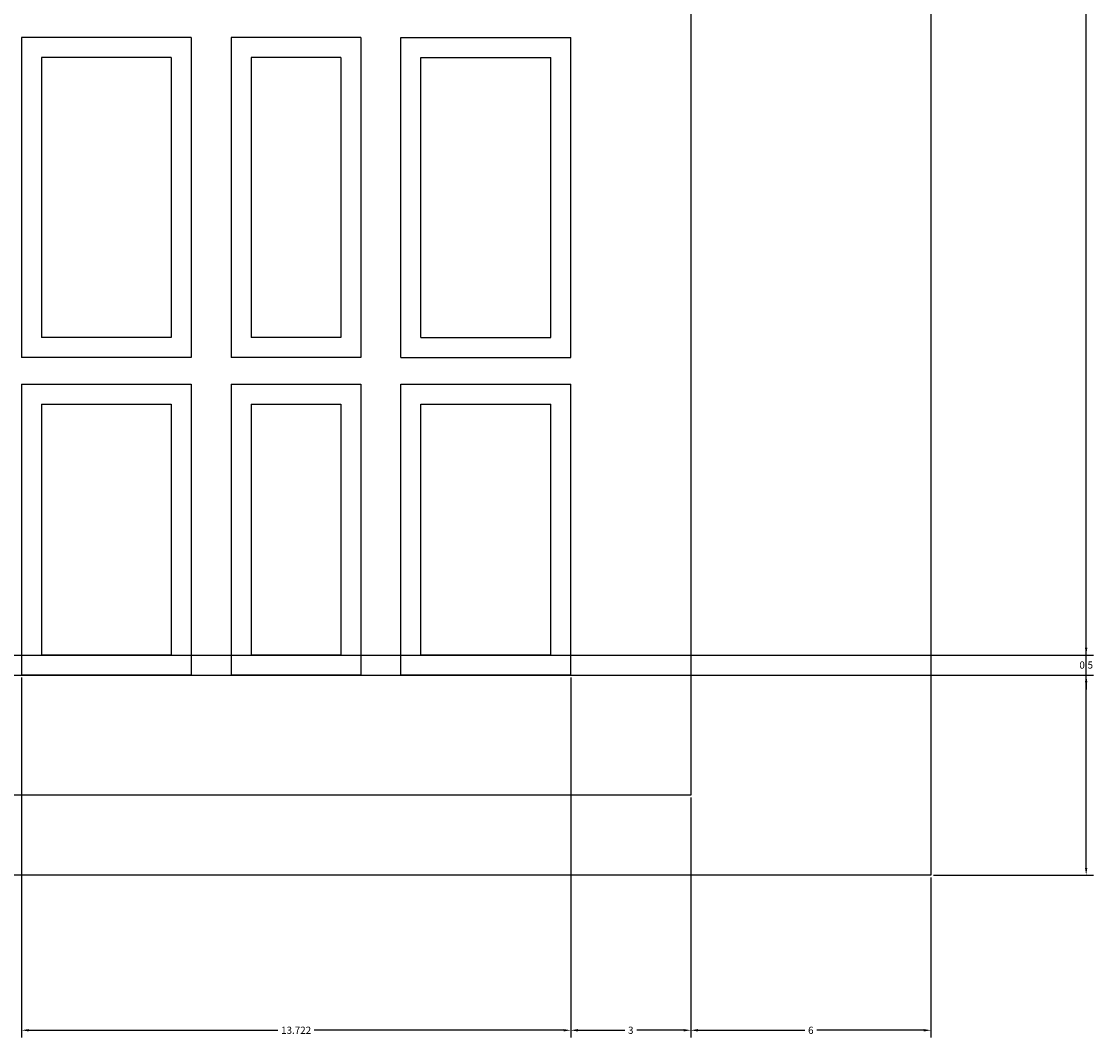
# Model space of a CAD drawing. Units: inches. Extents: x 12532.3 to 12594.9, y 6967.5 to 7063.
# Tile 4 of 9: x 12566.2 to 12593.1, y 6967.5 to 6992.9. Entities that reach past the tile are written whole.
import ezdxf

# ---------------------------------------------------------------- set-up
doc = ezdxf.new("R2010")
doc.units = ezdxf.units.IN
doc.header["$MEASUREMENT"] = 0
doc.header["$PDMODE"] = 98
doc.layers.add('A-ANNO-DIMS', color=2, linetype='Continuous', lineweight=18)
doc.layers.add('A-DOOR', color=4, linetype='Continuous', lineweight=25)
doc.styles.get("Standard").update_dxf_attribs({"font": 'arial.ttf'})
doc.dimstyles.get("Standard").update_dxf_attribs({"dimtxt": 0.18, "dimasz": 0.18, "dimexe": 0.18, "dimexo": 0.0625, "dimgap": 0.09, "dimtad": 0, "dimtih": 1, "dimtoh": 1, "dimdec": 4, "dimzin": 0, "dimdsep": 46, "dimtxsty": 'Standard', "dimcen": 0.09, "dimadec": 0, "dimazin": 0, "dimtfac": 1, "dimtdec": 4, "dimtofl": 0, "dimtmove": 0, "dimatfit": 3, "dimfxl": 1, "dimtolj": 1, "dimtzin": 0, "dimarcsym": 0})

# ---------------------------------------------------------------- blocks, each defined once
blk = doc.blocks.new('DOOR-PANEL-3_2x7_3')
for p, q in [((0, 7.273), (0, 0)), ((0, 7.273), (3.24, 7.273)), ((3.24, 7.273), (3.24, 0)), ((0.5, 6.773), (0.5, 0.5)), ((0.5, 6.773), (2.74, 6.773)), ((2.74, 6.773), (2.74, 0.5)), ((2.74, 0.5), (0.5, 0.5)), ((3.24, 0), (0, 0))]:
    blk.add_line(p, q)
blk = doc.blocks.new('DOOR-PANEL-4_2x7_3')
for p, q in [((0, 7.273), (0, 0)), ((0, 7.273), (4.241, 7.273)), ((4.241, 7.273), (4.241, 0)), ((0.5, 6.773), (0.5, 0.5)), ((0.5, 6.773), (3.741, 6.773)), ((3.741, 6.773), (3.741, 0.5)), ((3.741, 0.5), (0.5, 0.5)), ((4.241, 0), (0, 0))]:
    blk.add_line(p, q)
blk = doc.blocks.new('DOOR-PANEL-4_2x8_0')
for p, q in [((4.241, 8.003), (0, 8.003)), ((0, 8.003), (0, 0)), ((4.241, 8.003), (4.241, 0)), ((3.741, 7.503), (0.5, 7.503)), ((0.5, 7.503), (0.5, 0.5)), ((3.741, 7.503), (3.741, 0.5)), ((3.741, 0.5), (0.5, 0.5)), ((4.241, 0), (0, 0))]:
    blk.add_line(p, q)
blk = doc.blocks.new('DOOR-PANEL-3_2x8_0')
for p, q in [((3.24, 8.003), (0, 8.003)), ((0, 8.003), (0, 0)), ((3.24, 8.003), (3.24, 0)), ((2.74, 7.503), (0.5, 7.503)), ((0.5, 7.503), (0.5, 0.5)), ((2.74, 7.503), (2.74, 0.5)), ((2.74, 0.5), (0.5, 0.5)), ((3.24, 0), (0, 0))]:
    blk.add_line(p, q)
blk = doc.blocks.new('*D32')
at = {"layer": 'A-ANNO-DIMS', "color": 0, "lineweight": -2, "transparency": 16777216}
for p, q in [((12588.956, 7020.929), (12592.954, 7020.929)), ((12592.774, 7020.749), (12592.774, 6996.445)), ((12592.774, 6971.777), (12592.774, 6996.081)), ((12588.956, 6971.597), (12592.954, 6971.597))]:
    blk.add_line(p, q, dxfattribs=at)
at = {"layer": 'A-ANNO-DIMS', "color": 0, "transparency": 16777216}
for points in [[(12592.744, 7020.749), (12592.804, 7020.749), (12592.774, 7020.929)], [(12592.744, 6971.777), (12592.804, 6971.777), (12592.774, 6971.597)]]:
    blk.add_solid(points, dxfattribs=at)
at = {"layer": 'Defpoints', "color": 0, "transparency": 16777216}
for p in [(12588.894, 7020.929), (12592.774, 7020.929), (12588.894, 6971.597)]:
    blk.add_point(p, dxfattribs=at)
at = {"layer": 'A-ANNO-DIMS', "color": 0, "transparency": 16777216, "insert": (12592.774, 6996.263), "char_height": 0.18, "attachment_point": 5}
blk.add_mtext('\\A1;49.33', dxfattribs=at)
blk = doc.blocks.new('*D38')
at = {"layer": 'A-ANNO-DIMS', "color": 0, "lineweight": -2, "transparency": 16777216}
for p, q in [((12566.172, 6976.534), (12566.172, 6967.537)), ((12579.894, 6976.534), (12579.894, 6967.537)), ((12566.352, 6967.717), (12572.579, 6967.717)), ((12579.714, 6967.717), (12573.487, 6967.717))]:
    blk.add_line(p, q, dxfattribs=at)
at = {"layer": 'A-ANNO-DIMS', "color": 0, "transparency": 16777216}
for points in [[(12566.352, 6967.747), (12566.352, 6967.687), (12566.172, 6967.717)], [(12579.714, 6967.747), (12579.714, 6967.687), (12579.894, 6967.717)]]:
    blk.add_solid(points, dxfattribs=at)
at = {"layer": 'Defpoints', "color": 0, "transparency": 16777216}
for p in [(12566.172, 6976.597), (12579.894, 6976.597), (12579.894, 6967.717)]:
    blk.add_point(p, dxfattribs=at)
at = {"layer": 'A-ANNO-DIMS', "color": 0, "transparency": 16777216, "insert": (12573.033, 6967.717), "char_height": 0.18, "attachment_point": 5}
blk.add_mtext('\\A1;13.722', dxfattribs=at)
blk = doc.blocks.new('*D39')
at = {"layer": 'A-ANNO-DIMS', "color": 0, "lineweight": -2, "transparency": 16777216}
for p, q in [((12579.894, 6976.534), (12579.894, 6967.537)), ((12582.894, 6973.534), (12582.894, 6967.537)), ((12580.074, 6967.717), (12581.245, 6967.717)), ((12582.714, 6967.717), (12581.543, 6967.717))]:
    blk.add_line(p, q, dxfattribs=at)
at = {"layer": 'A-ANNO-DIMS', "color": 0, "transparency": 16777216}
for points in [[(12580.074, 6967.747), (12580.074, 6967.687), (12579.894, 6967.717)], [(12582.714, 6967.747), (12582.714, 6967.687), (12582.894, 6967.717)]]:
    blk.add_solid(points, dxfattribs=at)
at = {"layer": 'Defpoints', "color": 0, "transparency": 16777216}
for p in [(12579.894, 6976.597), (12582.894, 6973.597), (12582.894, 6967.717)]:
    blk.add_point(p, dxfattribs=at)
at = {"layer": 'A-ANNO-DIMS', "color": 0, "transparency": 16777216, "insert": (12581.394, 6967.717), "char_height": 0.18, "attachment_point": 5}
blk.add_mtext('\\A1;3', dxfattribs=at)
blk = doc.blocks.new('*D40')
at = {"layer": 'A-ANNO-DIMS', "color": 0, "lineweight": -2, "transparency": 16777216}
for p, q in [((12582.893999, 6973.534253), (12582.893999, 6967.536753)), ((12588.893999, 6971.534253), (12588.893999, 6967.536753)), ((12583.073999, 6967.716753), (12585.744572, 6967.716753)), ((12588.713999, 6967.716753), (12586.043426, 6967.716753))]:
    blk.add_line(p, q, dxfattribs=at)
at = {"layer": 'A-ANNO-DIMS', "color": 0, "transparency": 16777216}
for points in [[(12583.073999, 6967.746753), (12583.073999, 6967.686753), (12582.893999, 6967.716753)], [(12588.713999, 6967.746753), (12588.713999, 6967.686753), (12588.893999, 6967.716753)]]:
    blk.add_solid(points, dxfattribs=at)
at = {"layer": 'Defpoints', "color": 0, "transparency": 16777216}
for p in [(12582.893999, 6973.596753), (12588.893999, 6971.596753), (12588.893999, 6967.716753)]:
    blk.add_point(p, dxfattribs=at)
at = {"layer": 'A-ANNO-DIMS', "color": 0, "transparency": 16777216, "insert": (12585.893999, 6967.716753), "char_height": 0.18, "attachment_point": 5}
blk.add_mtext('\\A1;6', dxfattribs=at)
blk = doc.blocks.new('*D61')
at = {"layer": 'A-ANNO-DIMS', "color": 0, "lineweight": -2, "transparency": 16777216}
for p, q in [((12592.773999, 6977.276753), (12592.773999, 6977.456753)), ((12558.734573, 6977.096753), (12592.953999, 6977.096753)), ((12559.234573, 6976.596753), (12592.953999, 6976.596753)), ((12592.773999, 6976.416753), (12592.773999, 6976.236753))]:
    blk.add_line(p, q, dxfattribs=at)
at = {"layer": 'A-ANNO-DIMS', "color": 0, "transparency": 16777216}
for points in [[(12592.743999, 6977.276753), (12592.803999, 6977.276753), (12592.773999, 6977.096753)], [(12592.743999, 6976.416753), (12592.803999, 6976.416753), (12592.773999, 6976.596753)]]:
    blk.add_solid(points, dxfattribs=at)
at = {"layer": 'Defpoints', "color": 0, "transparency": 16777216}
for p in [(12558.672073, 6977.096753), (12592.773999, 6977.096753), (12559.172073, 6976.596753)]:
    blk.add_point(p, dxfattribs=at)
at = {"layer": 'A-ANNO-DIMS', "color": 0, "transparency": 16777216, "insert": (12592.773999, 6976.846753), "char_height": 0.18, "attachment_point": 5}
blk.add_mtext('\\A1;0.5', dxfattribs=at)

msp = doc.modelspace()

# ---------------------------------------------------------------- linework, layer by layer
at = {"layer": 'A-DOOR'}
msp.add_lwpolyline([(12536.4501, 7020.9287), (12588.894, 7020.9287), (12588.894, 6971.5968), (12536.4501, 6971.5968)], close=True, dxfattribs=at)
for points in [[(12582.894, 7018.9287), (12582.894, 6973.5968)], [(12582.894, 6973.5968), (12542.4501, 6973.5968)]]:
    msp.add_lwpolyline(points, dxfattribs=at)

# ---------------------------------------------------------------- block references
for name, p in [('DOOR-PANEL-4_2x8_0', (12566.1719, 6984.532)), ('DOOR-PANEL-3_2x8_0', (12571.4129, 6984.532)), ('DOOR-PANEL-4_2x7_3', (12566.1719, 6976.597)), ('DOOR-PANEL-3_2x7_3', (12571.4129, 6976.597))]:
    msp.add_blockref(name, p, dxfattribs=at)
at = {"layer": 'A-DOOR', "rotation": 180}
for name, p in [('DOOR-PANEL-4_2x8_0', (12579.8941, 6992.535)), ('DOOR-PANEL-4_2x7_3', (12579.8941, 6983.87))]:
    msp.add_blockref(name, p, dxfattribs=at)

# ---------------------------------------------------------------- dimensions: what is measured, and where the dimension line sits
at = {"layer": 'A-ANNO-DIMS'}
for base, p1, p2, override, picture, middle in [((12592.774, 7020.9287), (12588.894, 6971.5968), (12588.894, 7020.9287), {"dimdec": 2, "dimlfac": 1, "dimrnd": 0, "dimzin": 0, "dimdsep": 46, "dimlunit": 2}, '*D32', (12592.774, 6996.2627)), ((12592.774, 6977.0968), (12559.1721, 6976.5968), (12558.6721, 6977.0968), {"dimdec": 1, "dimlfac": 1, "dimrnd": 0, "dimzin": 0, "dimdsep": 46, "dimlunit": 2}, '*D61', (12592.774, 6976.8468))]:
    dim = msp.add_linear_dim(base=base, p1=p1, p2=p2, angle=90, dimstyle='Standard', override=override, dxfattribs=at)
    dim.commit()
    dim.dimension.update_dxf_attribs({"geometry": picture, "text_midpoint": middle})
for base, p1, p2, override, picture, middle in [((12579.894, 6967.7168), (12566.1721, 6976.5968), (12579.894, 6976.5968), {"dimdec": 3, "dimlfac": 1, "dimrnd": 0, "dimzin": 0, "dimdsep": 46, "dimlunit": 2}, '*D38', (12573.033, 6967.7168)), ((12582.894, 6967.7168), (12579.894, 6976.5968), (12582.894, 6973.5968), {"dimdec": 0, "dimlfac": 1, "dimrnd": 0, "dimzin": 0, "dimdsep": 46, "dimlunit": 2}, '*D39', (12581.394, 6967.7168)), ((12588.894, 6967.7168), (12582.894, 6973.5968), (12588.894, 6971.5968), {"dimdec": 0, "dimlfac": 1, "dimrnd": 0, "dimzin": 0, "dimdsep": 46, "dimlunit": 2}, '*D40', (12585.894, 6967.7168))]:
    dim = msp.add_linear_dim(base=base, p1=p1, p2=p2, dimstyle='Standard', override=override, dxfattribs=at)
    dim.commit()
    dim.dimension.update_dxf_attribs({"geometry": picture, "text_midpoint": middle})

doc.saveas('drawing.dxf')
